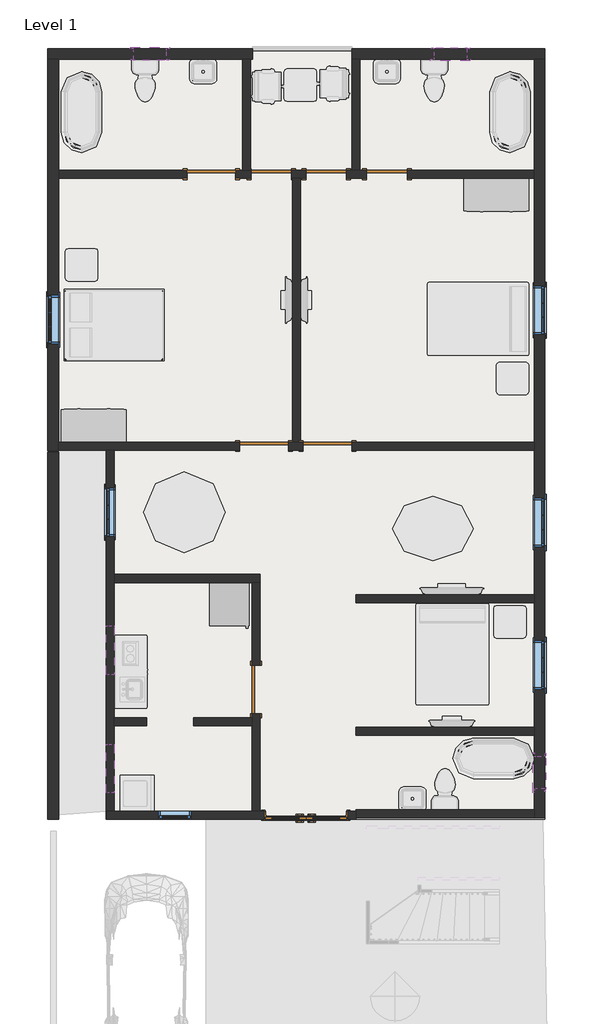
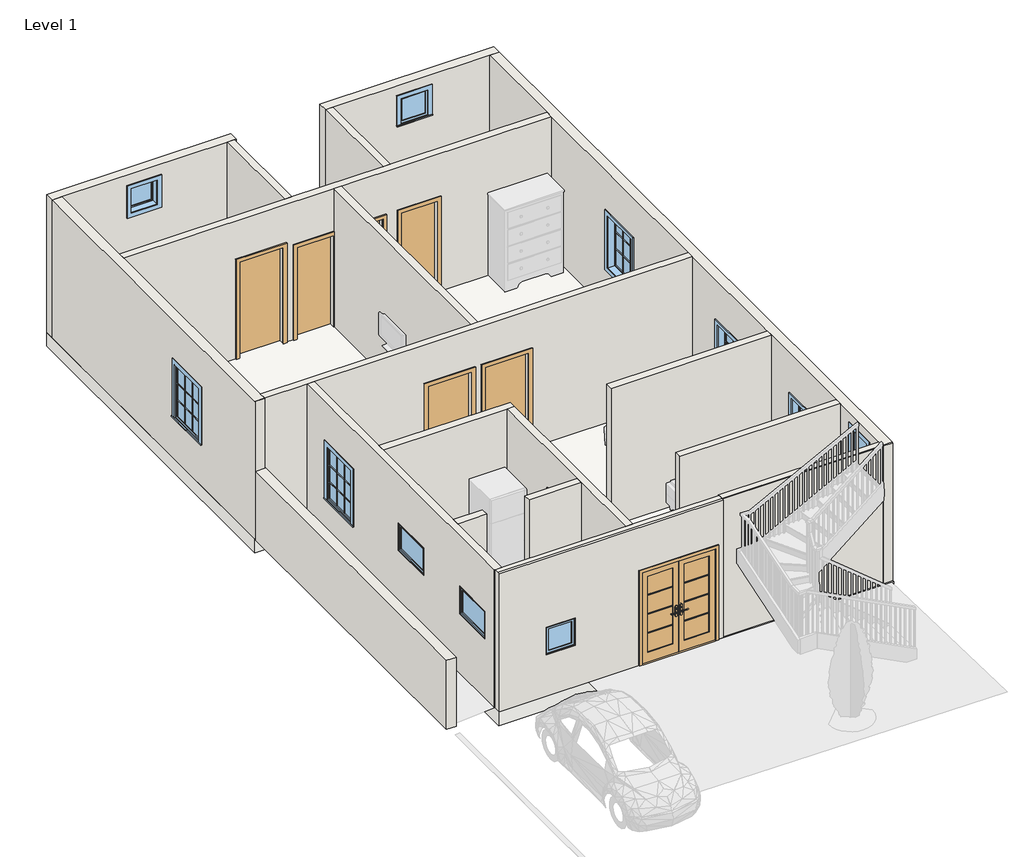
# One storey, part 1 of 3: 19 walls, 11 windows, 8 doors, 1 slab.
"""IFC4 building model written with IfcOpenShell, lengths in millimetres."""

from ifc_helpers import new_model, si_unit, frame, origin, origin_with_axes, place, context, project, spatial, polyline, outline, extrude, faceted_brep, transform, mapped, element, save
from components import door_94998e6c, door_255cab33, door_059fdd7e, door_16372e1c, door_686f89d2, window_29c06734, window_5c190c7e, window_aff1bc2a, window_fef7ae9c, window_e41d21a6

model = new_model("IFC4")

# Units and contexts
model_context = context("Model", 3, world=origin())
ifc_project = project(units=[si_unit("LENGTHUNIT", "METRE", prefix="MILLI")], contexts=[model_context])

# Site, building, storey
site = spatial("IfcSite", under=ifc_project)
building = spatial("IfcBuilding", under=site)
storey = spatial("IfcBuildingStorey", under=building, Name="Level 1", Elevation=0.0)

# Doors
placement = place(None, origin())
door_shape = door_94998e6c(model_context)
element("IfcDoor", 1, ObjectType="Door-Exterior-Double-Full Glass-Wood_Clad : 60\" x 80\"", at=placement, inside=storey, context=model_context, shape_type="MappedRepresentation", body=[
    mapped(door_shape, transform((-7061.4247577, -35.021371, 0.0), x_axis=(-1.0, 0.0, 0.0), y_axis=(0.0, -1.0, 0.0), z_axis=(0.0, 0.0, 1.0))),
])
door_2_shape = door_255cab33(model_context)
element("IfcDoor", 2, ObjectType="Single-Flush : 30\" x 80\"", at=placement, inside=storey, context=model_context, shape_type="MappedRepresentation", body=[
    mapped(door_2_shape, transform((-7709.1247577, 12007.753629, 0.0), x_axis=(-1.0, 0.0, 0.0), y_axis=(0.0, -1.0, 0.0), z_axis=(0.0, 0.0, 1.0))),
])
element("IfcDoor", 3, ObjectType="Single-Flush : 30\" x 80\"", at=placement, inside=storey, context=model_context, shape_type="MappedRepresentation", body=[
    mapped(door_2_shape, transform((-5537.4247577, 12007.753629, 0.0), x_axis=(-1.0, 0.0, 0.0), y_axis=(0.0, -1.0, 0.0), z_axis=(0.0, 0.0, 1.0))),
])
door_3_shape = door_059fdd7e(model_context)
element("IfcDoor", 4, ObjectType="Single-Flush : 30\" x 80\"", at=placement, inside=storey, context=model_context, shape_type="MappedRepresentation", body=[
    mapped(door_3_shape, transform((-6680.4247577, 12007.753629, 0.0), x_axis=(1.0, 0.0, 0.0), y_axis=(0.0, 1.0, 0.0), z_axis=(0.0, 0.0, 1.0))),
])
door_4_shape = door_16372e1c(model_context)
element("IfcDoor", 5, ObjectType="Single-Flush : 36\" x 84\"", at=placement, inside=storey, context=model_context, shape_type="MappedRepresentation", body=[
    mapped(door_4_shape, transform((-8839.4247577, 12007.753629, 0.0), x_axis=(1.0, 0.0, 0.0), y_axis=(0.0, 1.0, 0.0), z_axis=(0.0, 0.0, 1.0))),
])
element("IfcDoor", 6, ObjectType="Single-Flush : 36\" x 84\"", at=placement, inside=storey, context=model_context, shape_type="MappedRepresentation", body=[
    mapped(door_4_shape, transform((-7848.8247577, 6902.353629, 0.0), x_axis=(1.0, 0.0, 0.0), y_axis=(0.0, 1.0, 0.0), z_axis=(0.0, 0.0, 1.0))),
])
door_5_shape = door_686f89d2(model_context)
element("IfcDoor", 7, ObjectType="Single-Flush : 36\" x 84\"", at=placement, inside=storey, context=model_context, shape_type="MappedRepresentation", body=[
    mapped(door_5_shape, transform((-6655.0247577, 6902.353629, 0.0), x_axis=(-1.0, 0.0, 0.0), y_axis=(0.0, -1.0, 0.0), z_axis=(0.0, 0.0, 1.0))),
])
element("IfcDoor", 8, ObjectType="Single-Flush : 36\" x 84\"", at=placement, inside=storey, context=model_context, shape_type="MappedRepresentation", body=[
    mapped(door_5_shape, transform((-8001.2247577, 2330.353629, 0.0), x_axis=(0.0, -1.0, 0.0), y_axis=(1.0, 0.0, 0.0), z_axis=(0.0, 0.0, 1.0))),
])

# Slab
element("IfcSlab", 9, ObjectType="Generic - 12\"", at=placement, inside=storey, context=model_context, shape_type="SweptSolid", body=[
    extrude(outline(polyline([(-2565.6247577, 14369.953629), (-2565.6247577, -108.046371), (-10820.6247577, -108.046371), (-10820.6247577, 6826.153629), (-11912.8247577, 6826.153629), (-11912.8247577, 14369.953629), (-2565.6247577, 14369.953629)])), frame((0.0, 0.0, -304.8), z_axis=(0.0, 0.0, 1.0), x_axis=(1.0, 0.0, 0.0)), (0.0, 0.0, 1.0), 304.8),
])

# Walls
element("IfcWall", 10, ObjectType="Generic - 8\"", at=placement, inside=storey, context=model_context, shape_type="Brep", body=[
    faceted_brep([(-11912.8247577, 14166.753629, 0.0), (-11709.6247577, 14166.753629, 0.0), (-8255.2247577, 14166.753629, 0.0), (-8102.8247577, 14166.753629, 0.0), (-8064.7247577, 14166.753629, 0.0), (-8064.7247577, 14166.753629, 3048.0), (-8102.8247577, 14166.753629, 3048.0), (-8255.2247577, 14166.753629, 3048.0), (-11709.6247577, 14166.753629, 3048.0), (-11912.8247577, 14166.753629, 3048.0), (-9690.3247577, 14166.753629, 2768.6), (-9690.3247577, 14166.753629, 2159.0), (-10299.9247577, 14166.753629, 2159.0), (-10299.9247577, 14166.753629, 2768.6), (-11912.8247577, 14369.953629, 0.0), (-11912.8247577, 14369.953629, 3048.0), (-8064.7247577, 14369.953629, 3048.0), (-8064.7247577, 14369.953629, 0.0), (-9690.3247577, 14369.953629, 2768.6), (-10299.9247577, 14369.953629, 2768.6), (-10299.9247577, 14369.953629, 2159.0), (-9690.3247577, 14369.953629, 2159.0)], [[[0, 1, 2, 3, 4, 5, 6, 7, 8, 9], [10, 11, 12, 13]], [[14, 15, 16, 17], [18, 19, 20, 21]], [[4, 3, 2, 1, 0, 14, 17]], [[5, 4, 17, 16]], [[0, 9, 15, 14]], [[11, 10, 18, 21]], [[12, 11, 21, 20]], [[13, 12, 20, 19]], [[10, 13, 19, 18]], [[9, 8, 7, 6, 5, 16, 15]]]),
])
element("IfcWall", 11, ObjectType="Generic - 8\"", at=placement, inside=storey, context=model_context, shape_type="Brep", body=[
    faceted_brep([(-2768.8247577, 14166.753629, 0.0), (-2768.8247577, 12083.953629, 0.0), (-2768.8247577, 11931.553629, 0.0), (-2768.8247577, 6978.553629, 0.0), (-2768.8247577, 6826.153629, 0.0), (-2768.8247577, 4108.353629, 0.0), (-2768.8247577, 3955.953629, 0.0), (-2768.8247577, 1619.153629, 0.0), (-2768.8247577, 1466.753629, 0.0), (-2768.8247577, 69.753629, 0.0), (-2768.8247577, -82.646371, 0.0), (-2768.8247577, -82.646371, 3048.0), (-2768.8247577, -57.246371, 3048.0), (-2768.8247577, 69.753629, 3048.0), (-2768.8247577, 1466.753629, 3048.0), (-2768.8247577, 1619.153629, 3048.0), (-2768.8247577, 3955.953629, 3048.0), (-2768.8247577, 4108.353629, 3048.0), (-2768.8247577, 6826.153629, 3048.0), (-2768.8247577, 6978.553629, 3048.0), (-2768.8247577, 11931.553629, 3048.0), (-2768.8247577, 12083.953629, 3048.0), (-2768.8247577, 14166.753629, 3048.0), (-2768.8247577, 8997.853629, 2133.6), (-2768.8247577, 8997.853629, 914.4), (-2768.8247577, 9912.253629, 914.4), (-2768.8247577, 9912.253629, 2133.6), (-2768.8247577, 2330.353629, 2133.6), (-2768.8247577, 2330.353629, 914.4), (-2768.8247577, 3244.753629, 914.4), (-2768.8247577, 3244.753629, 2133.6), (-2768.8247577, 5010.053629, 2133.6), (-2768.8247577, 5010.053629, 914.4), (-2768.8247577, 5924.453629, 914.4), (-2768.8247577, 5924.453629, 2133.6), (-2768.8247577, 1073.053629, 2768.6), (-2768.8247577, 463.453629, 2768.6), (-2768.8247577, 463.453629, 2159.0), (-2768.8247577, 1073.053629, 2159.0), (-2565.6247577, 14166.753629, 0.0), (-2565.6247577, 14166.753629, 3048.0), (-2565.6247577, -57.246371, 3048.0), (-2565.6247577, -82.646371, 3048.0), (-2565.6247577, -82.646371, 0.0), (-2565.6247577, 8997.853629, 2133.6), (-2565.6247577, 9912.253629, 2133.6), (-2565.6247577, 9912.253629, 914.4), (-2565.6247577, 8997.853629, 914.4), (-2565.6247577, 2330.353629, 2133.6), (-2565.6247577, 3244.753629, 2133.6), (-2565.6247577, 3244.753629, 914.4), (-2565.6247577, 2330.353629, 914.4), (-2565.6247577, 5010.053629, 2133.6), (-2565.6247577, 5924.453629, 2133.6), (-2565.6247577, 5924.453629, 914.4), (-2565.6247577, 5010.053629, 914.4), (-2565.6247577, 1073.053629, 2768.6), (-2565.6247577, 1073.053629, 2159.0), (-2565.6247577, 463.453629, 2159.0), (-2565.6247577, 463.453629, 2768.6)], [[[0, 1, 2, 3, 4, 5, 6, 7, 8, 9, 10, 11, 12, 13, 14, 15, 16, 17, 18, 19, 20, 21, 22], [23, 24, 25, 26], [27, 28, 29, 30], [31, 32, 33, 34], [35, 36, 37, 38]], [[39, 40, 41, 42, 43], [44, 45, 46, 47], [48, 49, 50, 51], [52, 53, 54, 55], [56, 57, 58, 59]], [[10, 9, 8, 7, 6, 5, 4, 3, 2, 1, 0, 39, 43]], [[0, 22, 40, 39]], [[11, 10, 43, 42]], [[24, 23, 44, 47]], [[25, 24, 47, 46]], [[26, 25, 46, 45]], [[23, 26, 45, 44]], [[28, 27, 48, 51]], [[29, 28, 51, 50]], [[30, 29, 50, 49]], [[27, 30, 49, 48]], [[32, 31, 52, 55]], [[33, 32, 55, 54]], [[34, 33, 54, 53]], [[31, 34, 53, 52]], [[57, 56, 35, 38]], [[58, 57, 38, 37]], [[59, 58, 37, 36]], [[56, 59, 36, 35]], [[12, 11, 42, 41]], [[22, 21, 20, 19, 18, 17, 16, 15, 14, 13, 12, 41, 40]]]),
])
element("IfcWall", 12, ObjectType="Generic - 8\"", at=placement, inside=storey, context=model_context, shape_type="Brep", body=[
    faceted_brep([(-6197.8247577, 14166.753629, 0.0), (-6045.4247577, 14166.753629, 0.0), (-2768.8247577, 14166.753629, 0.0), (-2565.6247577, 14166.753629, 0.0), (-2565.6247577, 14166.753629, 3048.0), (-2768.8247577, 14166.753629, 3048.0), (-6045.4247577, 14166.753629, 3048.0), (-6197.8247577, 14166.753629, 3048.0), (-4648.4247577, 14166.753629, 2768.6), (-4038.8247577, 14166.753629, 2768.6), (-4038.8247577, 14166.753629, 2159.0), (-4648.4247577, 14166.753629, 2159.0), (-6197.8247577, 14369.953629, 0.0), (-6197.8247577, 14369.953629, 3048.0), (-2565.6247577, 14369.953629, 3048.0), (-2565.6247577, 14369.953629, 0.0), (-4648.4247577, 14369.953629, 2768.6), (-4648.4247577, 14369.953629, 2159.0), (-4038.8247577, 14369.953629, 2159.0), (-4038.8247577, 14369.953629, 2768.6)], [[[0, 1, 2, 3, 4, 5, 6, 7], [8, 9, 10, 11]], [[12, 13, 14, 15], [16, 17, 18, 19]], [[3, 2, 1, 0, 12, 15]], [[0, 7, 13, 12]], [[4, 3, 15, 14]], [[16, 19, 9, 8]], [[19, 18, 10, 9]], [[18, 17, 11, 10]], [[17, 16, 8, 11]], [[7, 6, 5, 4, 14, 13]]]),
])
element("IfcWall", 13, ObjectType="Generic - 8\"", at=placement, inside=storey, context=model_context, shape_type="SweptSolid", body=[
    extrude(outline(polyline([(-11709.6247577, 6788.053629), (-11709.6247577, -108.046371), (-11912.8247577, -108.046371), (-11912.8247577, 6788.053629), (-11709.6247577, 6788.053629)])), origin_with_axes(), (0.0, 0.0, 1.0), 1524.0),
])
element("IfcWall", 14, ObjectType="Generic - 8\"", at=placement, inside=storey, context=model_context, shape_type="Brep", body=[
    faceted_brep([(-11709.6247577, 6813.453629, 0.0), (-11709.6247577, 6826.153629, 0.0), (-11709.6247577, 6978.553629, 0.0), (-11709.6247577, 11931.553629, 0.0), (-11709.6247577, 12083.953629, 0.0), (-11709.6247577, 14166.753629, 0.0), (-11709.6247577, 14166.753629, 3048.0), (-11709.6247577, 12083.953629, 3048.0), (-11709.6247577, 11931.553629, 3048.0), (-11709.6247577, 6978.553629, 3048.0), (-11709.6247577, 6826.153629, 3048.0), (-11709.6247577, 6813.453629, 3048.0), (-11709.6247577, 9734.453629, 2133.6), (-11709.6247577, 9734.453629, 914.4), (-11709.6247577, 8820.053629, 914.4), (-11709.6247577, 8820.053629, 2133.6), (-11912.8247577, 6813.453629, 0.0), (-11912.8247577, 6813.453629, 3048.0), (-11912.8247577, 6826.153629, 3048.0), (-11912.8247577, 14166.753629, 3048.0), (-11912.8247577, 14166.753629, 0.0), (-11912.8247577, 9734.453629, 2133.6), (-11912.8247577, 8820.053629, 2133.6), (-11912.8247577, 8820.053629, 914.4), (-11912.8247577, 9734.453629, 914.4)], [[[0, 1, 2, 3, 4, 5, 6, 7, 8, 9, 10, 11], [12, 13, 14, 15]], [[16, 17, 18, 19, 20], [21, 22, 23, 24]], [[5, 4, 3, 2, 1, 0, 16, 20]], [[0, 11, 17, 16]], [[6, 5, 20, 19]], [[12, 15, 22, 21]], [[15, 14, 23, 22]], [[14, 13, 24, 23]], [[13, 12, 21, 24]], [[11, 10, 18, 17]], [[10, 9, 8, 7, 6, 19, 18]]]),
])
element("IfcWall", 15, ObjectType="INNER 6\"", at=placement, inside=storey, context=model_context, shape_type="Brep", body=[
    faceted_brep([(-6299.4247577, 11931.553629, 0.0), (-5918.4247577, 11931.553629, 0.0), (-5918.4247577, 11931.553629, 2032.0), (-5156.4247577, 11931.553629, 2032.0), (-5156.4247577, 11931.553629, 0.0), (-2768.8247577, 11931.553629, 0.0), (-2768.8247577, 11931.553629, 3048.0), (-7163.0247577, 11931.553629, 3048.0), (-7315.4247577, 11931.553629, 3048.0), (-11709.6247577, 11931.553629, 3048.0), (-11709.6247577, 11931.553629, 0.0), (-9296.6247577, 11931.553629, 0.0), (-9296.6247577, 11931.553629, 2133.6), (-8382.2247577, 11931.553629, 2133.6), (-8382.2247577, 11931.553629, 0.0), (-8090.1247577, 11931.553629, 0.0), (-8090.1247577, 11931.553629, 2032.0), (-7328.1247577, 11931.553629, 2032.0), (-7328.1247577, 11931.553629, 0.0), (-7315.4247577, 11931.553629, 0.0), (-7163.0247577, 11931.553629, 0.0), (-7061.4247577, 11931.553629, 0.0), (-7061.4247577, 11931.553629, 2032.0), (-6299.4247577, 11931.553629, 2032.0), (-5918.4247577, 12083.953629, 2032.0), (-5918.4247577, 12083.953629, 0.0), (-6045.4247577, 12083.953629, 0.0), (-6197.8247577, 12083.953629, 0.0), (-6299.4247577, 12083.953629, 0.0), (-6299.4247577, 12083.953629, 2032.0), (-7061.4247577, 12083.953629, 2032.0), (-7061.4247577, 12083.953629, 0.0), (-7328.1247577, 12083.953629, 0.0), (-7328.1247577, 12083.953629, 2032.0), (-8090.1247577, 12083.953629, 2032.0), (-8090.1247577, 12083.953629, 0.0), (-8102.8247577, 12083.953629, 0.0), (-8255.2247577, 12083.953629, 0.0), (-8382.2247577, 12083.953629, 0.0), (-8382.2247577, 12083.953629, 2133.6), (-9296.6247577, 12083.953629, 2133.6), (-9296.6247577, 12083.953629, 0.0), (-11709.6247577, 12083.953629, 0.0), (-11709.6247577, 12083.953629, 3048.0), (-8255.2247577, 12083.953629, 3048.0), (-8102.8247577, 12083.953629, 3048.0), (-6197.8247577, 12083.953629, 3048.0), (-6045.4247577, 12083.953629, 3048.0), (-2768.8247577, 12083.953629, 3048.0), (-2768.8247577, 12083.953629, 0.0), (-5156.4247577, 12083.953629, 0.0), (-5156.4247577, 12083.953629, 2032.0)], [[[0, 1, 2, 3, 4, 5, 6, 7, 8, 9, 10, 11, 12, 13, 14, 15, 16, 17, 18, 19, 20, 21, 22, 23]], [[24, 25, 26, 27, 28, 29, 30, 31, 32, 33, 34, 35, 36, 37, 38, 39, 40, 41, 42, 43, 44, 45, 46, 47, 48, 49, 50, 51]], [[11, 10, 42, 41]], [[38, 37, 36, 35, 15, 14]], [[21, 20, 19, 18, 32, 31]], [[50, 49, 5, 4]], [[28, 27, 26, 25, 1, 0]], [[10, 9, 43, 42]], [[6, 5, 49, 48]], [[39, 38, 14, 13]], [[40, 39, 13, 12]], [[41, 40, 12, 11]], [[16, 15, 35, 34]], [[17, 16, 34, 33]], [[18, 17, 33, 32]], [[29, 28, 0, 23]], [[30, 29, 23, 22]], [[31, 30, 22, 21]], [[2, 1, 25, 24]], [[3, 2, 24, 51]], [[4, 3, 51, 50]], [[9, 8, 7, 6, 48, 47, 46, 45, 44, 43]]]),
])
element("IfcWall", 16, ObjectType="INNER 6\"", at=placement, inside=storey, context=model_context, shape_type="SweptSolid", body=[
    extrude(outline(polyline([(-8102.8247577, 14166.753629), (-8102.8247577, 12083.953629), (-8255.2247577, 12083.953629), (-8255.2247577, 14166.753629), (-8102.8247577, 14166.753629)])), origin_with_axes(), (0.0, 0.0, 1.0), 3048.0),
])
element("IfcWall", 17, ObjectType="INNER 6\"", at=placement, inside=storey, context=model_context, shape_type="SweptSolid", body=[
    extrude(outline(polyline([(-6045.4247577, 14166.753629), (-6045.4247577, 12083.953629), (-6197.8247577, 12083.953629), (-6197.8247577, 14166.753629), (-6045.4247577, 14166.753629)])), origin_with_axes(), (0.0, 0.0, 1.0), 3048.0),
])
element("IfcWall", 18, ObjectType="INNER 6\"", at=placement, inside=storey, context=model_context, shape_type="SweptSolid", body=[
    extrude(outline(polyline([(-7315.4247577, 6978.553629), (-7315.4247577, 11931.553629), (-7163.0247577, 11931.553629), (-7163.0247577, 6978.553629), (-7315.4247577, 6978.553629)])), origin_with_axes(), (0.0, 0.0, 1.0), 3048.0),
])
element("IfcWall", 19, ObjectType="INNER 6\"", at=placement, inside=storey, context=model_context, shape_type="Brep", body=[
    faceted_brep([(-7112.2247577, 6978.553629, 2133.6), (-7112.2247577, 6978.553629, 0.0), (-7163.0247577, 6978.553629, 0.0), (-7315.4247577, 6978.553629, 0.0), (-7391.6247577, 6978.553629, 0.0), (-7391.6247577, 6978.553629, 2133.6), (-8306.0247577, 6978.553629, 2133.6), (-8306.0247577, 6978.553629, 0.0), (-11709.6247577, 6978.553629, 0.0), (-11709.6247577, 6978.553629, 3048.0), (-7315.4247577, 6978.553629, 3048.0), (-7163.0247577, 6978.553629, 3048.0), (-2768.8247577, 6978.553629, 3048.0), (-2768.8247577, 6978.553629, 0.0), (-6197.8247577, 6978.553629, 0.0), (-6197.8247577, 6978.553629, 2133.6), (-7391.6247577, 6826.153629, 0.0), (-7112.2247577, 6826.153629, 0.0), (-7112.2247577, 6826.153629, 2133.6), (-6197.8247577, 6826.153629, 2133.6), (-6197.8247577, 6826.153629, 0.0), (-2768.8247577, 6826.153629, 0.0), (-2768.8247577, 6826.153629, 3048.0), (-10668.2247577, 6826.153629, 3048.0), (-10820.6247577, 6826.153629, 3048.0), (-11709.6247577, 6826.153629, 3048.0), (-11709.6247577, 6826.153629, 0.0), (-10820.6247577, 6826.153629, 0.0), (-10668.2247577, 6826.153629, 0.0), (-8306.0247577, 6826.153629, 0.0), (-8306.0247577, 6826.153629, 2133.6), (-7391.6247577, 6826.153629, 2133.6)], [[[0, 1, 2, 3, 4, 5, 6, 7, 8, 9, 10, 11, 12, 13, 14, 15]], [[16, 17, 18, 19, 20, 21, 22, 23, 24, 25, 26, 27, 28, 29, 30, 31]], [[29, 28, 27, 26, 8, 7]], [[14, 13, 21, 20]], [[4, 3, 2, 1, 17, 16]], [[9, 8, 26, 25]], [[13, 12, 22, 21]], [[5, 4, 16, 31]], [[6, 5, 31, 30]], [[7, 6, 30, 29]], [[18, 17, 1, 0]], [[19, 18, 0, 15]], [[20, 19, 15, 14]], [[12, 11, 10, 9, 25, 24, 23, 22]]]),
])
element("IfcWall", 20, ObjectType="INNER 6\"", at=placement, inside=storey, context=model_context, shape_type="Brep", body=[
    faceted_brep([(-10820.6247577, 6826.153629, 0.0), (-10820.6247577, 44.353629, 0.0), (-10820.6247577, 44.353629, 3048.0), (-10820.6247577, 6826.153629, 3048.0), (-10820.6247577, 6114.953629, 2133.6), (-10820.6247577, 5200.553629, 2133.6), (-10820.6247577, 5200.553629, 914.4), (-10820.6247577, 6114.953629, 914.4), (-10820.6247577, 3524.153629, 1981.2), (-10820.6247577, 2609.753629, 1981.2), (-10820.6247577, 2609.753629, 1371.6), (-10820.6247577, 3524.153629, 1371.6), (-10820.6247577, 1301.653629, 1930.4), (-10820.6247577, 387.253629, 1930.4), (-10820.6247577, 387.253629, 1320.8), (-10820.6247577, 1301.653629, 1320.8), (-10668.2247577, 6826.153629, 0.0), (-10668.2247577, 6826.153629, 3048.0), (-10668.2247577, 4489.353629, 3048.0), (-10668.2247577, 4336.953629, 3048.0), (-10668.2247577, 1796.953629, 3048.0), (-10668.2247577, 1644.553629, 3048.0), (-10668.2247577, 44.353629, 3048.0), (-10668.2247577, 44.353629, 0.0), (-10668.2247577, 1644.553629, 0.0), (-10668.2247577, 1796.953629, 0.0), (-10668.2247577, 4336.953629, 0.0), (-10668.2247577, 4489.353629, 0.0), (-10668.2247577, 6114.953629, 2133.6), (-10668.2247577, 6114.953629, 914.4), (-10668.2247577, 5200.553629, 914.4), (-10668.2247577, 5200.553629, 2133.6), (-10668.2247577, 3524.153629, 1981.2), (-10668.2247577, 3524.153629, 1371.6), (-10668.2247577, 2609.753629, 1371.6), (-10668.2247577, 2609.753629, 1981.2), (-10668.2247577, 1301.653629, 1930.4), (-10668.2247577, 1301.653629, 1320.8), (-10668.2247577, 387.253629, 1320.8), (-10668.2247577, 387.253629, 1930.4), (-10807.9247577, 44.353629, 0.0), (-10807.9247577, 44.353629, 3048.0)], [[[0, 1, 2, 3], [4, 5, 6, 7], [8, 9, 10, 11], [12, 13, 14, 15]], [[16, 17, 18, 19, 20, 21, 22, 23, 24, 25, 26, 27], [28, 29, 30, 31], [32, 33, 34, 35], [36, 37, 38, 39]], [[1, 0, 16, 27, 26, 25, 24, 23, 40]], [[0, 3, 17, 16]], [[2, 1, 40, 23, 22, 41]], [[29, 28, 4, 7]], [[30, 29, 7, 6]], [[31, 30, 6, 5]], [[28, 31, 5, 4]], [[33, 32, 8, 11]], [[34, 33, 11, 10]], [[35, 34, 10, 9]], [[32, 35, 9, 8]], [[37, 36, 12, 15]], [[38, 37, 15, 14]], [[39, 38, 14, 13]], [[36, 39, 13, 12]], [[3, 2, 41, 22, 21, 20, 19, 18, 17]]]),
])
element("IfcWall", 21, ObjectType="INNER 6\"", at=placement, inside=storey, context=model_context, shape_type="Brep", body=[
    faceted_brep([(-10807.9247577, 44.353629, 0.0), (-10807.9247577, 44.353629, 3048.0), (-10668.2247577, 44.353629, 3048.0), (-8077.4247577, 44.353629, 3048.0), (-7925.0247577, 44.353629, 3048.0), (-6121.6247577, 44.353629, 3048.0), (-6121.6247577, 44.353629, 0.0), (-6274.0247577, 44.353629, 0.0), (-6274.0247577, 44.353629, 2057.4), (-7848.8247577, 44.353629, 2057.4), (-7848.8247577, 44.353629, 0.0), (-7925.0247577, 44.353629, 0.0), (-8077.4247577, 44.353629, 0.0), (-10668.2247577, 44.353629, 0.0), (-9830.0247577, 44.353629, 1524.0), (-9830.0247577, 44.353629, 914.4), (-9220.4247577, 44.353629, 914.4), (-9220.4247577, 44.353629, 1524.0), (-10807.9247577, -108.046371, 3048.0), (-10807.9247577, -108.046371, 0.0), (-7848.8247577, -108.046371, 0.0), (-7848.8247577, -108.046371, 2057.4), (-6274.0247577, -108.046371, 2057.4), (-6274.0247577, -108.046371, 0.0), (-6121.6247577, -108.046371, 0.0), (-6121.6247577, -108.046371, 3048.0), (-9830.0247577, -108.046371, 1524.0), (-9220.4247577, -108.046371, 1524.0), (-9220.4247577, -108.046371, 914.4), (-9830.0247577, -108.046371, 914.4), (-6121.6247577, -82.646371, 0.0), (-10807.9247577, -57.246371, 3048.0), (-6121.6247577, -57.246371, 3048.0), (-6121.6247577, -82.646371, 3048.0)], [[[0, 1, 2, 3, 4, 5, 6, 7, 8, 9, 10, 11, 12, 13], [14, 15, 16, 17]], [[18, 19, 20, 21, 22, 23, 24, 25], [26, 27, 28, 29]], [[19, 0, 13, 12, 11, 10, 20]], [[6, 30, 24, 23, 7]], [[1, 0, 19, 18, 31]], [[6, 5, 32, 33, 25, 24, 30]], [[9, 21, 20, 10]], [[21, 9, 8, 22]], [[22, 8, 7, 23]], [[15, 14, 26, 29]], [[16, 15, 29, 28]], [[17, 16, 28, 27]], [[14, 17, 27, 26]], [[18, 25, 33, 32, 31]], [[5, 4, 3, 2, 1, 31, 32]]]),
])
element("IfcWall", 22, ObjectType="INNER 6\"", at=placement, inside=storey, context=model_context, shape_type="Brep", body=[
    faceted_brep([(-7925.0247577, 4489.353629, 0.0), (-10668.2247577, 4489.353629, 0.0), (-10668.2247577, 4489.353629, 3048.0), (-7925.0247577, 4489.353629, 3048.0), (-7925.0247577, 4336.953629, 0.0), (-7925.0247577, 4336.953629, 3048.0), (-8077.4247577, 4336.953629, 3048.0), (-10668.2247577, 4336.953629, 3048.0), (-10668.2247577, 4336.953629, 0.0), (-8077.4247577, 4336.953629, 0.0)], [[[0, 1, 2, 3]], [[4, 5, 6, 7, 8, 9]], [[1, 0, 4, 9, 8]], [[2, 1, 8, 7]], [[0, 3, 5, 4]], [[3, 2, 7, 6, 5]]]),
])
element("IfcWall", 23, ObjectType="INNER 6\"", at=placement, inside=storey, context=model_context, shape_type="Brep", body=[
    faceted_brep([(-8077.4247577, 1873.153629, 2133.6), (-8077.4247577, 1873.153629, 0.0), (-8077.4247577, 1796.953629, 0.0), (-8077.4247577, 1644.553629, 0.0), (-8077.4247577, 44.353629, 0.0), (-8077.4247577, 44.353629, 3048.0), (-8077.4247577, 1644.553629, 3048.0), (-8077.4247577, 1796.953629, 3048.0), (-8077.4247577, 4336.953629, 3048.0), (-8077.4247577, 4336.953629, 0.0), (-8077.4247577, 2787.553629, 0.0), (-8077.4247577, 2787.553629, 2133.6), (-7925.0247577, 44.353629, 0.0), (-7925.0247577, 1873.153629, 0.0), (-7925.0247577, 1873.153629, 2133.6), (-7925.0247577, 2787.553629, 2133.6), (-7925.0247577, 2787.553629, 0.0), (-7925.0247577, 4336.953629, 0.0), (-7925.0247577, 4336.953629, 3048.0), (-7925.0247577, 44.353629, 3048.0)], [[[0, 1, 2, 3, 4, 5, 6, 7, 8, 9, 10, 11]], [[12, 13, 14, 15, 16, 17, 18, 19]], [[10, 9, 17, 16]], [[4, 3, 2, 1, 13, 12]], [[5, 4, 12, 19]], [[9, 8, 18, 17]], [[14, 13, 1, 0]], [[15, 14, 0, 11]], [[16, 15, 11, 10]], [[8, 7, 6, 5, 19, 18]]]),
])
element("IfcWall", 24, ObjectType="INNER 6\"", at=placement, inside=storey, context=model_context, shape_type="SweptSolid", body=[
    extrude(outline(polyline([(-10058.6247577, 1644.553629), (-10668.2247577, 1644.553629), (-10668.2247577, 1796.953629), (-10058.6247577, 1796.953629), (-10058.6247577, 1644.553629)])), origin_with_axes(), (0.0, 0.0, 1.0), 3048.0),
])
element("IfcWall", 25, ObjectType="INNER 6\"", at=placement, inside=storey, context=model_context, shape_type="SweptSolid", body=[
    extrude(outline(polyline([(-6121.6247577, 4108.353629), (-2768.8247577, 4108.353629), (-2768.8247577, 3955.953629), (-6121.6247577, 3955.953629), (-6121.6247577, 4108.353629)])), origin_with_axes(), (0.0, 0.0, 1.0), 3048.0),
])
element("IfcWall", 26, ObjectType="INNER 6\"", at=placement, inside=storey, context=model_context, shape_type="SweptSolid", body=[
    extrude(outline(polyline([(-2768.8247577, 1466.753629), (-6121.6247577, 1466.753629), (-6121.6247577, 1619.153629), (-2768.8247577, 1619.153629), (-2768.8247577, 1466.753629)])), origin_with_axes(), (0.0, 0.0, 1.0), 3048.0),
])
element("IfcWall", 27, ObjectType="INNER 6\"", at=placement, inside=storey, context=model_context, shape_type="Brep", body=[
    faceted_brep([(-2768.8247577, 69.753629, 0.0), (-6121.6247577, 69.753629, 0.0), (-6121.6247577, 69.753629, 3048.0), (-2768.8247577, 69.753629, 3048.0), (-2768.8247577, -82.646371, 0.0), (-2768.8247577, -82.646371, 3048.0), (-6121.6247577, -82.646371, 3048.0), (-6121.6247577, -82.646371, 0.0), (-6121.6247577, 44.353629, 0.0), (-6121.6247577, -57.246371, 3048.0), (-6121.6247577, 44.353629, 3048.0), (-2768.8247577, -57.246371, 3048.0)], [[[0, 1, 2, 3]], [[4, 5, 6, 7]], [[1, 0, 4, 7, 8]], [[2, 1, 8, 7, 6, 9, 10]], [[0, 3, 11, 5, 4]], [[9, 6, 5, 11]], [[3, 2, 10, 9, 11]]]),
])
element("IfcWall", 28, ObjectType="INNER 6\"", at=placement, inside=storey, context=model_context, shape_type="SweptSolid", body=[
    extrude(outline(polyline([(-8077.4247577, 1644.553629), (-9169.6247577, 1644.553629), (-9169.6247577, 1796.953629), (-8077.4247577, 1796.953629), (-8077.4247577, 1644.553629)])), origin_with_axes(), (0.0, 0.0, 1.0), 3048.0),
])

# Windows
window_shape = window_29c06734(model_context)
element("IfcWindow", 29, ObjectType="Casement 3x3 with Trim : 36\" x 48\"", at=placement, inside=storey, context=model_context, shape_type="MappedRepresentation", body=[
    mapped(window_shape, transform((-11811.2247577, 9277.253629, 0.0), x_axis=(0.0, 1.0, 0.0), y_axis=(-1.0, 0.0, 0.0), z_axis=(0.0, 0.0, 1.0))),
])
element("IfcWindow", 30, ObjectType="Casement 3x3 with Trim : 36\" x 48\"", at=placement, inside=storey, context=model_context, shape_type="MappedRepresentation", body=[
    mapped(window_shape, transform((-2667.2247577, 9455.053629, 0.0), x_axis=(0.0, -1.0, 0.0), y_axis=(1.0, 0.0, 0.0), z_axis=(0.0, 0.0, 1.0))),
])
element("IfcWindow", 31, ObjectType="Casement 3x3 with Trim : 36\" x 48\"", at=placement, inside=storey, context=model_context, shape_type="MappedRepresentation", body=[
    mapped(window_shape, transform((-2667.2247577, 2787.553629, 0.0), x_axis=(0.0, -1.0, 0.0), y_axis=(1.0, 0.0, 0.0), z_axis=(0.0, 0.0, 1.0))),
])
element("IfcWindow", 32, ObjectType="Casement 3x3 with Trim : 36\" x 48\"", at=placement, inside=storey, context=model_context, shape_type="MappedRepresentation", body=[
    mapped(window_shape, transform((-2667.2247577, 5467.253629, 0.0), x_axis=(0.0, -1.0, 0.0), y_axis=(1.0, 0.0, 0.0), z_axis=(0.0, 0.0, 1.0))),
])
window_2_shape = window_5c190c7e(model_context)
element("IfcWindow", 33, ObjectType="Casement 3x3 with Trim : 36\" x 48\"", at=placement, inside=storey, context=model_context, shape_type="MappedRepresentation", body=[
    mapped(window_2_shape, transform((-10744.4247577, 5657.753629, 0.0), x_axis=(0.0, 1.0, 0.0), y_axis=(-1.0, 0.0, 0.0), z_axis=(0.0, 0.0, 1.0))),
])
window_3_shape = window_aff1bc2a(model_context)
element("IfcWindow", 34, ObjectType="Fixed : 24\" x 24\"", at=placement, inside=storey, context=model_context, shape_type="MappedRepresentation", body=[
    mapped(window_3_shape, transform((-9563.3247577, -31.846371, 0.0), x_axis=(-1.0, 0.0, 0.0), y_axis=(0.0, -1.0, 0.0), z_axis=(0.0, 0.0, 1.0))),
])
window_4_shape = window_fef7ae9c(model_context)
element("IfcWindow", 35, ObjectType="Fixed : 36\" x 24\"", at=placement, inside=storey, context=model_context, shape_type="MappedRepresentation", body=[
    mapped(window_4_shape, transform((-10744.4247577, 3105.053629, 457.2), x_axis=(0.0, 1.0, 0.0), y_axis=(-1.0, 0.0, 0.0), z_axis=(0.0, 0.0, 1.0))),
])
element("IfcWindow", 36, ObjectType="Fixed : 36\" x 24\"", at=placement, inside=storey, context=model_context, shape_type="MappedRepresentation", body=[
    mapped(window_4_shape, transform((-10744.4247577, 882.553629, 406.4), x_axis=(0.0, 1.0, 0.0), y_axis=(-1.0, 0.0, 0.0), z_axis=(0.0, 0.0, 1.0))),
])
window_5_shape = window_e41d21a6(model_context)
element("IfcWindow", 37, ObjectType="Transom with Trim : 24\" x 24\"", at=placement, inside=storey, context=model_context, shape_type="MappedRepresentation", body=[
    mapped(window_5_shape, transform((-2667.2247577, 806.353629, 0.0), x_axis=(0.0, 1.0, 0.0), y_axis=(-1.0, 0.0, 0.0), z_axis=(0.0, 0.0, 1.0))),
])
element("IfcWindow", 38, ObjectType="Transom with Trim : 24\" x 24\"", at=placement, inside=storey, context=model_context, shape_type="MappedRepresentation", body=[
    mapped(window_5_shape, transform((-4381.7247577, 14268.353629, 0.0), x_axis=(-1.0, 0.0, 0.0), y_axis=(0.0, -1.0, 0.0), z_axis=(0.0, 0.0, 1.0))),
])
element("IfcWindow", 39, ObjectType="Transom with Trim : 24\" x 24\"", at=placement, inside=storey, context=model_context, shape_type="MappedRepresentation", body=[
    mapped(window_5_shape, transform((-9957.0247577, 14268.353629, 0.0), x_axis=(1.0, 0.0, 0.0), y_axis=(0.0, 1.0, 0.0), z_axis=(0.0, 0.0, 1.0))),
])

save(model, "model.ifc")

# Revit data of these elements
# Type "Door-Exterior-Double-Full Glass-Wood_Clad : 60\" x 80\""
#   Type Mark = "8"
#   Assembly Code = "B2030100"
#   Analytic Construction = "French door, wood frame with double glass"
#   Top Rail = 0' - 4 11/16"
#   Threshold Offset [instance default] = 0' - 0 1/2"
#   Thickness = 0' - 1 3/8"
#   Thermal Resistance (R) = 1.9158 (h·ft²·°F)/BTU
#   Swing Angle [instance default] = 90.00°
#   Stiles = 0' - 4 3/4"
#   Rough Width = 5' - 2"
#   Rough Height = 6' - 9"
#   Panel Width = 2' - 6"
#   Door Offset [instance default] = 0' - 0"
#   Height = 6' - 8"
#   Width = 5' - 0"
#   Heat Transfer Coefficient (U) = 0.5220 BTU/(h·ft²·°F)
#   Bottom Rail = 0' - 9 1/8"
#   Exterior Trim [instance default] = yes
#   Threshold [instance default] = yes
#   Show Grill [instance default] = yes
#   Function = 1
#   Trim Material = Cherry
#   Threshold Material = Cherry
#   Panel Material = Cherry
#   Glazing = Glass
#   Frame Material = Cherry
#   Door Handle Material = Aluminum
#   Visual Light Transmittance = 0
#   Solar Heat Gain Coefficient = 0
#   Wall Closure = (empty or 0)
#   Construction Type = (empty or 0)
# Type "Single-Flush : 30\" x 80\""
#   Type Mark = "5"
#   Construction Type Id = "MDOOR"
#   Assembly Code = "C1020"
#   Analytic Construction = "Metal"
#   Thickness = 0' - 2"
#   Heat Transfer Coefficient (U) = 0.651978 BTU/(h·ft²·°F)
#   Height = 6' - 8"
#   Trim Projection Ext = 0' - 1"
#   Trim Projection Int = 0' - 1"
#   Trim Width = 0' - 3"
#   Width = 2' - 6"
#   Define Thermal Properties by = 1
#   Door Material = Door - Panel
#   Frame Material = Door - Frame
#   Visual Light Transmittance = 0
#   Solar Heat Gain Coefficient = 0
#   Function = (empty or 0)
#   Wall Closure = (empty or 0)
# Type "Single-Flush : 36\" x 84\""
#   Type Mark = "1"
#   Construction Type Id = "MDOOR"
#   Assembly Code = "C1020"
#   Analytic Construction = "Metal"
#   Thickness = 0' - 2"
#   Heat Transfer Coefficient (U) = 0.651978 BTU/(h·ft²·°F)
#   Height = 7' - 0"
#   Trim Projection Ext = 0' - 1"
#   Trim Projection Int = 0' - 1"
#   Trim Width = 0' - 3"
#   Width = 3' - 0"
#   Define Thermal Properties by = 1
#   Door Material = Door - Panel
#   Frame Material = Door - Frame
#   Visual Light Transmittance = 0
#   Solar Heat Gain Coefficient = 0
#   Function = (empty or 0)
#   Wall Closure = (empty or 0)
# Type "Generic - 12\""
#   Assembly Code = "B1010"
#   Function = 0
#   Layers, outside or top first: 1' - 0" no material (function 1)
# Type "Generic - 8\""
#   Assembly Code = "B2010"
#   Layers, outside or top first: 0' - 8" "Brick, Common" (function 1)
# Type "INNER 6\""
#   Assembly Code = "B2010"
#   Layers, outside or top first: 0' - 6" "Brick, Common" (function 1)
# Type "Casement 3x3 with Trim : 36\" x 48\""
#   Type Mark = "10"
#   Construction Type Id = "GSP4R"
#   Assembly Code = "B2020100"
#   Analytic Construction = "1/8 in Pilkington single glazing"
#   Visual Light Transmittance = 0.9
#   Solar Heat Gain Coefficient = 0.78
#   Heat Transfer Coefficient (U) = 0.6496 BTU/(h·ft²·°F)
#   Height = 4' - 0"
#   Default Sill Height = 3' - 0"
#   Trim Projection - Ext. = 0' - 0 1/2"
#   Trim Projection - Int. = 0' - 0 3/4"
#   Trim Width - Exterior = 0' - 3 1/2"
#   Trim Width - Interior = 0' - 3 1/2"
#   Width = 3' - 0"
#   Window Inset = 0' - 0 3/4"
#   Define Thermal Properties by = 1
#   Glass Pane Material = Glass
#   Sash Material = Sash
#   Trim Exterior Material = Trim
#   Trim Interior Material = Trim
#   Wall Closure = (empty or 0)
# Type "Fixed : 24\" x 24\""
#   Type Mark = "3"
#   Construction Type Id = "GSP4R"
#   Assembly Code = "B2020100"
#   Analytic Construction = "1/8 in Pilkington single glazing"
#   Visual Light Transmittance = 0.9
#   Solar Heat Gain Coefficient = 0.78
#   Heat Transfer Coefficient (U) = 0.6496 BTU/(h·ft²·°F)
#   Height = 2' - 0"
#   Default Sill Height = 3' - 0"
#   Width = 2' - 0"
#   Window Inset = 0' - 0 3/4"
#   Define Thermal Properties by = 1
#   Glass Pane Material = Glass
#   Sash Material = Sash
#   Wall Closure = (empty or 0)
# Type "Fixed : 36\" x 24\""
#   Type Mark = "8"
#   Construction Type Id = "GSP4R"
#   Assembly Code = "B2020100"
#   Analytic Construction = "1/8 in Pilkington single glazing"
#   Visual Light Transmittance = 0.9
#   Solar Heat Gain Coefficient = 0.78
#   Heat Transfer Coefficient (U) = 0.6496 BTU/(h·ft²·°F)
#   Height = 2' - 0"
#   Default Sill Height = 3' - 0"
#   Width = 3' - 0"
#   Window Inset = 0' - 0 3/4"
#   Define Thermal Properties by = 1
#   Glass Pane Material = Glass
#   Sash Material = Sash
#   Wall Closure = (empty or 0)
# Type "Transom with Trim : 24\" x 24\""
#   Type Mark = "13"
#   Construction Type Id = "GSP4R"
#   Assembly Code = "B2020100"
#   Analytic Construction = "1/8 in Pilkington single glazing"
#   Visual Light Transmittance = 0.9
#   Solar Heat Gain Coefficient = 0.78
#   Heat Transfer Coefficient (U) = 0.6496 BTU/(h·ft²·°F)
#   Height = 2' - 0"
#   Default Sill Height = 7' - 1"
#   Trim Projection - Ext. = 0' - 0 1/2"
#   Trim Projection - Int. = 0' - 0 3/4"
#   Trim Width - Exterior = 0' - 3 1/2"
#   Trim Width - Interior = 0' - 3 1/2"
#   Width = 2' - 0"
#   Window Inset = 0' - 0 3/4"
#   Define Thermal Properties by = 1
#   Glass Pane Material = Glass
#   Sash Material = Sash
#   Trim Exterior Material = Trim
#   Trim Interior Material = Trim
#   Wall Closure = (empty or 0)
# Element 1 (IfcDoor, "Door-Exterior-Double-Full Glass-Wood_Clad : 60\" x 80\"")
#   Threshold Offset = 0' - 0 1/2"
#   Swing Angle = 90.00°
#   Door Offset = 0' - 0"
#   Threshold = yes
#   Show Grill = yes
#   Exterior Trim = yes
#   Phase Created = New Construction
#   Materials on its faces: "Cherry", "Aluminum", "Glass"
# Elements 2, 3, 4 (IfcDoor, "Single-Flush : 30\" x 80\"")
#   Phase Created = New Construction
#   Materials on its faces: "Door - Frame", "Door - Panel"
# Elements 5, 6, 7, 8 (IfcDoor, "Single-Flush : 36\" x 84\"")
#   Phase Created = New Construction
#   Materials on its faces: "Door - Frame", "Door - Panel"
# Element 9 (IfcSlab, "Generic - 12\"")
#   Height Offset From Level = 0' - 0"
#   Phase Created = New Construction
#   Materials on its faces: "Default Floor"
# Elements 10, 11, 12, 14 (IfcWall, "Generic - 8\"")
#   Top Offset = 0' - 0"
#   Base Offset = 0' - 0"
#   Unconnected Height = 10' - 0"
#   wall height = 10' - 0"
#   Phase Created = New Construction
#   Base Constraint = Level 1
#   Materials on its faces: "Brick, Common"
# Element 13 (IfcWall, "Generic - 8\"")
#   Top Offset = 0' - 0"
#   Base Offset = 0' - 0"
#   Unconnected Height = 5' - 0"
#   wall height = 5' - 0"
#   Phase Created = New Construction
#   Base Constraint = Level 1
#   Materials on its faces: "Brick, Common"
# Elements 15, 16, 17, 18, 19, 20, 21, 22, 23, 24, 25, 26, 27, 28 (IfcWall, "INNER 6\"")
#   Top Offset = 0' - 0"
#   Base Offset = 0' - 0"
#   Unconnected Height = 10' - 0"
#   wall height = 10' - 0"
#   Phase Created = New Construction
#   Base Constraint = Level 1
#   Materials on its faces: "Brick, Common"
# Element 29 (IfcWindow, "Casement 3x3 with Trim : 36\" x 48\"")
#   Mark = "1"
#   Phase Created = New Construction
#   Materials on its faces: "Sash", "Glass", "Trim"
# Element 30 (IfcWindow, "Casement 3x3 with Trim : 36\" x 48\"")
#   Mark = "2"
#   Phase Created = New Construction
#   Materials on its faces: "Sash", "Glass", "Trim"
# Element 31 (IfcWindow, "Casement 3x3 with Trim : 36\" x 48\"")
#   Mark = "4"
#   Phase Created = New Construction
#   Materials on its faces: "Sash", "Glass", "Trim"
# Element 32 (IfcWindow, "Casement 3x3 with Trim : 36\" x 48\"")
#   Mark = "5"
#   Phase Created = New Construction
#   Materials on its faces: "Sash", "Glass", "Trim"
# Element 33 (IfcWindow, "Casement 3x3 with Trim : 36\" x 48\"")
#   Mark = "3"
#   Phase Created = New Construction
#   Materials on its faces: "Sash", "Glass", "Trim"
# Element 34 (IfcWindow, "Fixed : 24\" x 24\"")
#   Mark = "11"
#   Phase Created = New Construction
#   Materials on its faces: "Sash", "Glass"
# Element 35 (IfcWindow, "Fixed : 36\" x 24\"")
#   Mark = "6"
#   Phase Created = New Construction
#   Materials on its faces: "Sash", "Glass"
# Element 36 (IfcWindow, "Fixed : 36\" x 24\"")
#   Mark = "7"
#   Phase Created = New Construction
#   Materials on its faces: "Sash", "Glass"
# Element 37 (IfcWindow, "Transom with Trim : 24\" x 24\"")
#   Mark = "8"
#   Phase Created = New Construction
#   Materials on its faces: "Sash", "Trim", "Glass"
# Element 38 (IfcWindow, "Transom with Trim : 24\" x 24\"")
#   Mark = "9"
#   Phase Created = New Construction
#   Materials on its faces: "Sash", "Trim", "Glass"
# Element 39 (IfcWindow, "Transom with Trim : 24\" x 24\"")
#   Mark = "10"
#   Phase Created = New Construction
#   Materials on its faces: "Sash", "Trim", "Glass"
# Materials
#   "Cherry": class "Wood", colour RGB 226 177 128, transparency 0, Description = "Prunus Serotina", Cost = 0
#   "Glass": class "Glass", colour RGB 0 128 192, transparency 0.75, Description = "Soda Lime Glass", Cost = 0
#   "Aluminum": class "Metal", colour RGB 247 247 247, transparency 0, Description = "Aluminum 6061", Cost = 0
#   "Door - Panel": class "Wood", colour RGB 210 159 95, transparency 0
#   "Door - Frame": colour RGB 118 70 51, transparency 0
#   "Brick, Common": class "Masonry", colour RGB 170 98 104, transparency 0, Description = "Common brick", Cost = 0
#   "Sash": class "Wood", colour RGB 224 178 126, transparency 0
#   "Trim": class "Wood", colour RGB 224 178 126, transparency 0
#   "Default Floor": colour RGB 128 128 128, transparency 0
# Room at (-10171.37, 13208.484) mm, phase "New Construction", upper level "Level 1", upper offset 10' - 0", lower offset 0' - 0"
#   Number = "1"
# Room at (-7107.666, 13782.928) mm, phase "New Construction", upper level "Level 1", upper offset 10' - 0", lower offset 0' - 0"
#   Number = "2"
#   Name = "OPEN SKY"
# Room at (-4554.579, 13208.484) mm, phase "New Construction", upper level "Level 1", upper offset 10' - 0", lower offset 0' - 0"
#   Number = "3"
# Room at (-9501.185, 9410.767) mm, phase "New Construction", upper level "Level 1", upper offset 10' - 0", lower offset 0' - 0"
#   Number = "4"
#   Name = "MASTER BEDROOM"
# Room at (-4554.579, 10144.78) mm, phase "New Construction", upper level "Level 1", upper offset 10' - 0", lower offset 0' - 0"
#   Number = "5"
#   Name = "MASTER BEDROOM"
# Room at (-11329.985, 4623.729) mm, phase "New Construction", upper level "Level 1", upper offset 10' - 0", lower offset 0' - 0"
#   Number = "6"
# Room at (-8936.466, 5885.885) mm, phase "New Construction", upper level "Level 1", upper offset 10' - 0", lower offset 0' - 0"
#   Number = "7"
#   Name = "DINING"
# Room at (-5278.866, 5885.885) mm, phase "New Construction", upper level "Level 1", upper offset 10' - 0", lower offset 0' - 0"
#   Number = "8"
#   Name = "LIVING"
# Room at (-8936.466, 3361.574) mm, phase "New Construction", upper level "Level 1", upper offset 10' - 0", lower offset 0' - 0"
#   Number = "9"
#   Name = "KITCHEN"
# Room at (-9501.185, 1017.494) mm, phase "New Construction", upper level "Level 1", upper offset 10' - 0", lower offset 0' - 0"
#   Number = "10"
#   Name = "WASHING"
# Room at (-4554.579, 3361.574) mm, phase "New Construction", upper level "Level 1", upper offset 10' - 0", lower offset 0' - 0"
#   Number = "11"
#   Name = "GUEST ROOM"
# Room at (-3948.221, 1017.494) mm, phase "New Construction", upper level "Level 1", upper offset 10' - 0", lower offset 0' - 0"
#   Number = "12"
# Room at (-10171.37, -2205.778) mm, phase "New Construction", upper level "Level 1", upper offset 10' - 0", lower offset 0' - 0"
#   Number = "13"
#   Name = "PARKING"
# Room at (-4554.579, -2780.223) mm, phase "New Construction", upper level "Level 1", upper offset 10' - 0", lower offset 0' - 0"
#   Number = "14"
#   Name = "LAWN"
# Room at (-4554.579, -943.623) mm, phase "New Construction", upper level "Level 1", upper offset 10' - 0", lower offset 0' - 0"
#   Number = "15"
#   Name = "STAIRS"
# Room at (-7107.666, -3467.934) mm, phase "New Construction", upper level "Level 1", upper offset 10' - 0", lower offset 0' - 0"
#   Number = "16"
#   Name = "ENTRANCE"
# Room at (-6944.326, 2904.374) mm, phase "New Construction", upper level "Level 1", upper offset 10' - 0", lower offset 0' - 0"
#   Number = "17"
#   Name = "FOYER"
